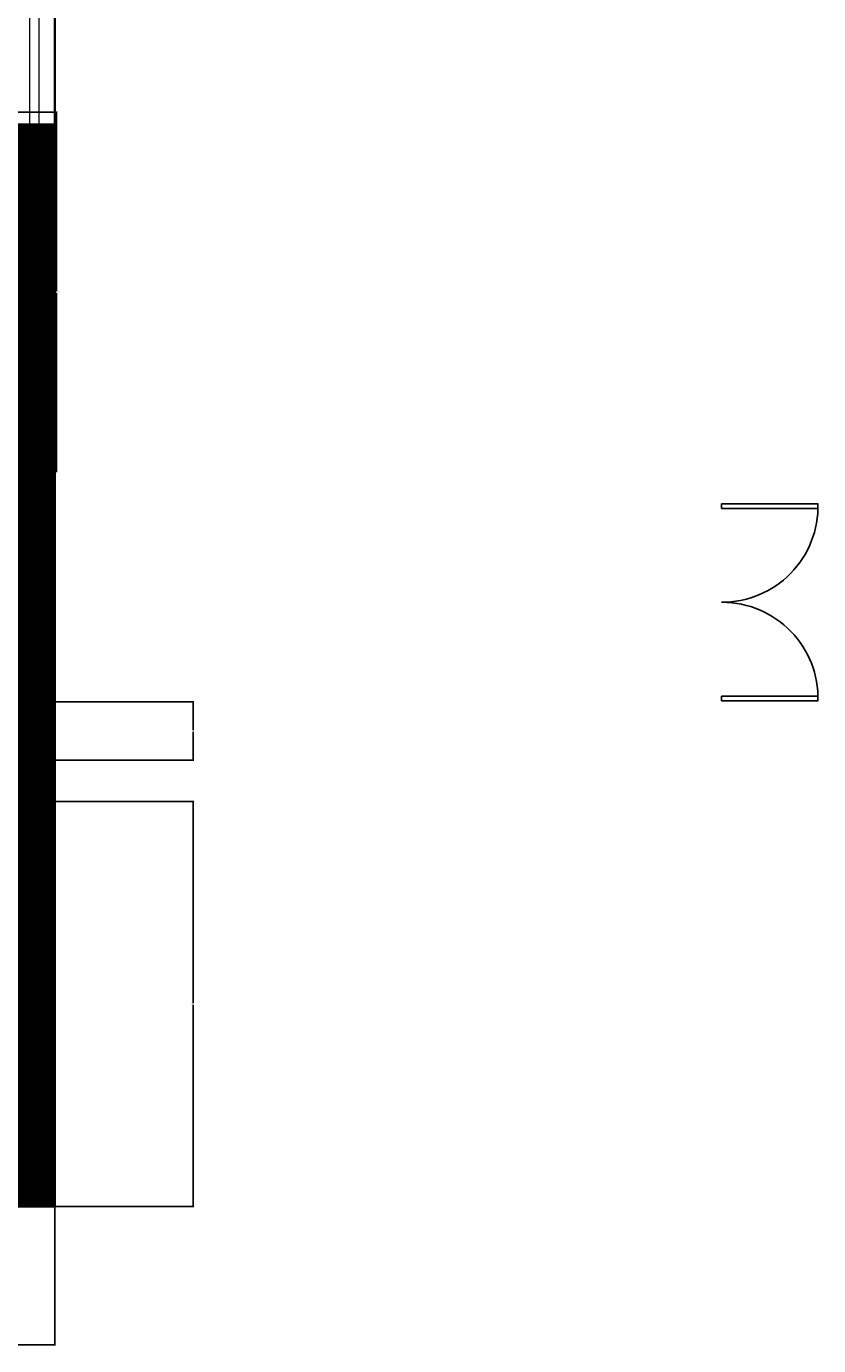
# Model space of a CAD drawing. Units: inches. Extents: x 205 to 1667, y -23 to 828.
# Tile 5 of 10: x 768 to 941, y -23 to 264. Entities that reach past the tile are written whole.
import ezdxf

# ---------------------------------------------------------------- set-up
doc = ezdxf.new("R2010")
doc.units = ezdxf.units.IN
doc.header["$MEASUREMENT"] = 0
for name, color, linetype, lineweight in [('A-ANNO-DIMS', 2, 'Continuous', 18), ('A-DOOR', 4, 'Continuous', 25), ('A-GLAZ', 4, 'Continuous', 18), ('A-WALL', 7, 'Continuous', 35)]:
    doc.layers.add(name, color=color, linetype=linetype, lineweight=lineweight)
doc.layers.add('A-FLOR-PATT', color=9, linetype='Continuous', lineweight=9, true_color=0xc7c8ca)
doc.styles.get("Standard").update_dxf_attribs({"font": 'arial.ttf'})
doc.dimstyles.get("Standard").update_dxf_attribs({"dimtxt": 0.18, "dimasz": 0.18, "dimexe": 0.18, "dimexo": 0.0625, "dimgap": 0.09, "dimtad": 0, "dimtih": 1, "dimtoh": 1, "dimdec": 4, "dimzin": 0, "dimdsep": 46, "dimtxsty": 'Standard', "dimcen": 0.09, "dimadec": 0, "dimazin": 0, "dimtfac": 1, "dimtdec": 4, "dimtofl": 0, "dimtmove": 0, "dimatfit": 3, "dimfxl": 1, "dimtolj": 1, "dimtzin": 0, "dimarcsym": 0})

# ---------------------------------------------------------------- blocks, each defined once
blk = doc.blocks.new('WIN-48IN')
for p, q in [((0, 0), (0, 9)), ((0, 9), (48, 9)), ((48, 9), (48, 0)), ((48, 5.5), (0, 5.5)), ((48, 3.5), (0, 3.5)), ((48, 0), (0, 0))]:
    blk.add_line(p, q)
blk = doc.blocks.new('DOOR-PAIR-21IN-LEAVES')
for p, q in [((0, 42.78), (0, 41.78)), ((0, 42.78), (21, 42.78)), ((0, 41.78), (21, 41.78)), ((0, 1), (0, 0)), ((0, 1), (21, 1)), ((0, 0), (21, 0))]:
    blk.add_line(p, q)
for centre, start, end in [((0.11, 42.28), 269.6873, 1.3714), ((0.11, 0.5), 358.6286, 89.6873)]:
    blk.add_arc(centre, 20.89, start, end)
blk = doc.blocks.new('*D38')
at = {"layer": 'A-ANNO-DIMS', "color": 0, "lineweight": -2, "transparency": 16777216}
for p, q in [((763.1, 245.49), (774.93, 245.49)), ((774.75, 245.31), (774.75, 206.61)), ((774.75, 167.53), (774.75, 206.24)), ((763.1, 167.35), (774.93, 167.35))]:
    blk.add_line(p, q, dxfattribs=at)
at = {"layer": 'A-ANNO-DIMS', "color": 0, "transparency": 16777216}
for points in [[(774.72, 245.31), (774.78, 245.31), (774.75, 245.49)], [(774.72, 167.53), (774.78, 167.53), (774.75, 167.35)]]:
    blk.add_solid(points, dxfattribs=at)
at = {"layer": 'Defpoints', "color": 0, "transparency": 16777216}
for p in [(763.03, 245.49), (763.03, 167.35), (774.75, 167.35)]:
    blk.add_point(p, dxfattribs=at)
at = {"layer": 'A-ANNO-DIMS', "color": 0, "transparency": 16777216, "insert": (774.75, 206.42), "char_height": 0.18, "attachment_point": 5}
blk.add_mtext('\\A1;SOFA 78', dxfattribs=at)
blk = doc.blocks.new('*D42')
at = {"layer": 'A-ANNO-DIMS', "color": 0, "lineweight": -2, "transparency": 16777216}
for p, q in [((462.43, 7.59), (462.43, -22.59)), ((774.43, 7.59), (774.43, -22.59)), ((462.61, -22.41), (618.14, -22.41)), ((774.25, -22.41), (618.72, -22.41))]:
    blk.add_line(p, q, dxfattribs=at)
at = {"layer": 'A-ANNO-DIMS', "color": 0, "transparency": 16777216}
for points in [[(462.61, -22.38), (462.61, -22.44), (462.43, -22.41)], [(774.25, -22.38), (774.25, -22.44), (774.43, -22.41)]]:
    blk.add_solid(points, dxfattribs=at)
at = {"layer": 'Defpoints', "color": 0, "transparency": 16777216}
for p in [(462.43, 7.65), (774.43, 7.65), (774.43, -22.41)]:
    blk.add_point(p, dxfattribs=at)
at = {"layer": 'A-ANNO-DIMS', "color": 0, "transparency": 16777216, "insert": (618.43, -22.41), "char_height": 0.18, "attachment_point": 5}
blk.add_mtext('\\A1;312', dxfattribs=at)
blk = doc.blocks.new('*D45')
at = {"layer": 'A-ANNO-DIMS', "color": 0, "lineweight": -2, "transparency": 16777216}
for p, q in [((765.49, 95.64), (804.67, 95.64)), ((804.49, 95.46), (804.49, 51.83)), ((804.49, 7.83), (804.49, 51.46)), ((774.49, 7.65), (804.67, 7.65))]:
    blk.add_line(p, q, dxfattribs=at)
at = {"layer": 'A-ANNO-DIMS', "color": 0, "transparency": 16777216}
for points in [[(804.46, 95.46), (804.52, 95.46), (804.49, 95.64)], [(804.46, 7.83), (804.52, 7.83), (804.49, 7.65)]]:
    blk.add_solid(points, dxfattribs=at)
at = {"layer": 'Defpoints', "color": 0, "transparency": 16777216}
for p in [(765.43, 95.64), (804.49, 95.64), (774.43, 7.65)]:
    blk.add_point(p, dxfattribs=at)
at = {"layer": 'A-ANNO-DIMS', "color": 0, "transparency": 16777216, "insert": (804.49, 51.64), "char_height": 0.18, "attachment_point": 5}
blk.add_mtext('\\A1;87.99', dxfattribs=at)
blk = doc.blocks.new('*D70')
at = {"layer": 'A-ANNO-DIMS', "color": 0, "lineweight": -2, "transparency": 16777216}
for p, q in [((729.04, 117.32), (804.67, 117.32)), ((804.49, 117.14), (804.49, 111.16)), ((804.49, 104.82), (804.49, 110.8)), ((765.49, 104.64), (804.67, 104.64))]:
    blk.add_line(p, q, dxfattribs=at)
at = {"layer": 'A-ANNO-DIMS', "color": 0, "transparency": 16777216}
for points in [[(804.46, 117.14), (804.52, 117.14), (804.49, 117.32)], [(804.46, 104.82), (804.52, 104.82), (804.49, 104.64)]]:
    blk.add_solid(points, dxfattribs=at)
at = {"layer": 'Defpoints', "color": 0, "transparency": 16777216}
for p in [(728.98, 117.32), (804.49, 117.32), (765.43, 104.64)]:
    blk.add_point(p, dxfattribs=at)
at = {"layer": 'A-ANNO-DIMS', "color": 0, "transparency": 16777216, "insert": (804.49, 110.98), "char_height": 0.18, "attachment_point": 5}
blk.add_mtext('\\A1;12.68', dxfattribs=at)

msp = doc.modelspace()

# ---------------------------------------------------------------- hatches: boundary and pattern name
at = {"layer": 'A-FLOR-PATT'}
h = msp.add_hatch(dxfattribs=at)
h.set_pattern_fill('ANSI31', color=256)
h.paths.add_polyline_path([(774.4305, 607.6511), (720.5338, 607.6511), (720.5338, 598.6511), (727.9933, 598.6511), (746.8614, 598.6511), (765.4305, 598.6511), (765.4305, 454.6511), (759.5298, 454.6511), (759.5298, 448.9635), (765.4305, 448.9635), (765.4305, 428.0602), (774.4305, 428.0602)])
h.paths.add_polyline_path([(765.4305, 598.6511), (746.8614, 598.6511), (746.8614, 579.7829), (727.9933, 579.7829), (727.9933, 518.1387, -0.41421701), (724.6389, 514.7843), (668.2693, 514.7843, -0.41421356), (665.0743, 517.9793), (665.0743, 579.7829), (646.2062, 579.7829), (646.2062, 598.6511), (626.3468, 598.6511), (626.3468, 454.6511), (628.3468, 454.6511), (628.3468, 484.9635, -0.41421356), (664.3468, 449.9635), (664.3468, 454.6511), (729.3305, 454.6511), (758.5298, 454.6511), (759.5298, 454.6511), (765.4305, 454.6511)])
h.paths.add_polyline_path([(621.4404, 598.6511), (471.4305, 598.6511), (471.4305, 568.8442), (490.2987, 568.8442), (490.2987, 549.9761), (551.9429, 549.9761, -0.41421701), (555.2973, 546.6217), (555.2973, 490.2521, -0.41421356), (552.1023, 487.0571), (490.2987, 487.0571), (490.2987, 468.189), (471.4305, 468.189), (471.4305, 454.6511), (583.4404, 454.6511), (583.4404, 449.9635, -0.41421356), (619.4404, 484.9635), (619.4404, 454.6511), (621.4404, 454.6511)])
h.paths.add_polyline_path([(672.5338, 607.6511), (569.5707, 607.6511), (569.5707, 598.6511), (621.4404, 598.6511), (621.4404, 454.6511), (619.4404, 454.6511), (619.4404, 448.9635), (628.3468, 448.9635), (628.3468, 454.6511), (626.3468, 454.6511), (626.3468, 598.6511), (646.2062, 598.6511), (665.0743, 598.6511), (672.5338, 598.6511)])
h.paths.add_polyline_path([(521.5707, 607.6511), (462.4305, 607.6511), (462.4305, 407.4306), (471.4305, 407.4306), (471.4305, 448.9635), (583.4404, 448.9635, -0.0070419), (583.4404, 449.9635), (583.4404, 454.6511), (471.4305, 454.6511), (471.4305, 468.189), (471.4305, 487.0571), (471.4305, 549.9761), (471.4305, 568.8442), (471.4305, 598.6511), (521.5707, 598.6511)])
h.paths.add_polyline_path([(471.4305, 314.3187), (583.4404, 314.3187), (583.4404, 319.9388), (471.4305, 319.9388), (471.4305, 359.4306), (462.4305, 359.4306), (462.4305, 7.6511), (471.4305, 7.6511), (471.4305, 204.9321), (521.9355, 204.9321), (521.9355, 213.9321), (471.4305, 213.9321)])
h.paths.add_polyline_path([(774.4305, 410.0602), (765.4305, 410.0602), (765.4305, 389.1569), (672.3024, 389.1569), (672.3024, 448.9635), (681.1739, 448.9635, -0.18532444), (681.6564, 449.1487), (698.6035, 449.1487), (729.3305, 448.9635), (729.3305, 454.6511), (664.3468, 454.6511), (664.3468, 449.9635, -0.0070419), (664.3468, 448.9635), (666.3024, 448.9635), (666.3024, 378.2485), (672.3024, 378.2485), (672.3024, 383.1306), (765.4305, 383.1306), (765.4305, 360.5347), (774.4305, 360.5347)])
h.paths.add_polyline_path([(774.4305, 342.5347), (765.4305, 342.5347), (765.4305, 319.9388), (672.3024, 319.9388), (672.3024, 348.5574), (671.0896, 348.5574, -0.04071533), (666.3024, 348.2485), (666.3024, 319.9388), (664.3468, 319.9388, -0.0070419), (664.3468, 318.9388), (664.3468, 314.3187), (765.4305, 314.3187), (765.4305, 290.8426), (774.4305, 290.8426)])
h.paths.add_polyline_path([(774.4305, 242.8426), (765.4305, 242.8426), (765.4305, 104.6382), (626.3468, 104.6382), (626.3468, 110.5917), (617.3468, 110.5917), (617.3468, 95.6382), (765.4305, 95.6382), (765.4305, 16.6511), (621.2232, 16.6511), (621.2232, 7.6511), (774.4305, 7.6511)])
h.paths.add_polyline_path([(626.3468, 314.3187), (628.3468, 314.3187), (628.3468, 319.9388), (619.4404, 319.9388), (619.4404, 314.3187), (620.4404, 314.3187), (620.4404, 213.9321), (569.9355, 213.9321), (569.9355, 204.9321), (617.3468, 204.9321), (617.3468, 153.3751), (626.3468, 153.3751)])
h.paths.add_polyline_path([(620.4404, 314.3187), (619.4404, 314.3187), (619.4404, 319.9388), (628.3468, 319.9388), (629.3468, 319.9388), (629.3468, 283.9388, 0.40598745), (664.3468, 318.9388), (664.3468, 319.9388), (666.3024, 319.9388), (666.3024, 348.2485), (666.3024, 377.2485), (666.3024, 378.2485), (666.3024, 448.9635), (664.3468, 448.9635), (664.3468, 449.9635, 0.40598745), (629.3468, 484.9635), (629.3468, 448.9635), (628.3468, 448.9635), (619.4404, 448.9635), (618.4404, 448.9635), (618.4404, 484.9635, 0.40598745), (583.4404, 449.9635), (583.4404, 448.9635), (471.4305, 448.9635), (471.4305, 407.4306), (471.4305, 359.4306), (471.4305, 319.9388), (583.4404, 319.9388), (583.4404, 314.3187), (495.4305, 314.3187), (495.4305, 237.9321), (620.4404, 237.9321)])
h.paths.add_polyline_path([(525.0876, 347.7863), (513.5657, 347.7863), (512.0216, 362.1672), (526.6317, 362.1672)], flags=16)
h.paths.add_polyline_path([(550.9499, 370.1471), (536.569, 368.6029), (536.569, 383.2131), (550.9499, 381.6689)], flags=16)
h.paths.add_polyline_path([(530.7713, 364.5431), (508.0415, 364.5431, -0.41421356), (504.7944, 367.7902), (504.7944, 403.5085, -0.41421356), (508.0415, 406.7556), (530.7713, 406.7556, -0.41421356), (534.0184, 403.5085), (534.0184, 367.7902, -0.41421356)], flags=16)
h.paths.add_polyline_path([(550.9499, 389.6298), (536.569, 388.0856), (536.569, 402.6958), (550.9499, 401.1516)], flags=16)
h.paths.add_polyline_path([(502.2439, 368.6029), (487.863, 370.1471), (487.863, 381.6689), (502.2439, 383.2131)], flags=16)
h.paths.add_polyline_path([(502.2439, 388.0856), (487.863, 389.6298), (487.863, 401.1516), (502.2439, 402.6958)], flags=16)
h.paths.add_polyline_path([(526.6317, 409.1315), (512.0216, 409.1315), (513.5657, 423.5124), (525.0876, 423.5124)], flags=16)
h.paths.add_polyline_path([(765.4305, 290.8426), (765.4305, 314.3187), (664.3468, 314.3187), (664.3468, 318.9388, -0.41421356), (628.3468, 283.9388), (628.3468, 314.3187), (626.3468, 314.3187), (626.3468, 153.3751), (638.3468, 153.3751, -0.4196361), (617.5748, 131.9834, -0.4196361), (638.3468, 110.5917), (626.3468, 110.5917), (626.3468, 104.6382), (765.4305, 104.6382), (765.4305, 242.8426)])
h.paths.add_polyline_path([(691.5064, 243.4363), (693.2483, 243.4363), (725.4984, 243.4363), (725.4984, 241.7329), (725.4984, 177.0512), (723.7564, 177.0512), (691.5064, 177.0512), (691.5064, 178.7545)], flags=16)
h.paths.add_polyline_path([(689.8658, 265.2977), (689.8658, 296.6873, -0.41421356), (690.8346, 297.6561), (724.6111, 297.6561, -0.41421356), (725.5799, 296.6873), (725.5799, 265.2977, -0.41421356), (724.6111, 264.3289), (690.8346, 264.3289, -0.41421356)], flags=16)
h.paths.add_polyline_path([(694.1286, 265.6852), (694.1286, 288.9368, -0.41421356), (695.0974, 289.9056), (720.3483, 289.9056, -0.41421356), (721.3171, 288.9368), (721.3171, 265.6852, -0.04533947), (721.3013, 265.5106, -0.3531705), (720.3282, 264.7164), (695.0974, 264.7164, -0.41421356)], flags=0)
h.paths.add_polyline_path([(694.1286, 291.2619), (694.1286, 294.7497, -0.41421356), (695.0974, 295.7185), (720.3483, 295.7185, -0.41421356), (721.3171, 294.7497), (721.3171, 291.2619, -0.41421356), (720.3483, 290.2931), (695.0974, 290.2931, -0.41421356)], flags=0)
h.paths.add_polyline_path([(734.4369, 244.6615, -0.41421356), (735.2682, 245.4928), (762.2019, 245.4928, -0.41421356), (763.0332, 244.6615), (763.0332, 168.183, -0.41421356), (762.2019, 167.3517), (735.2682, 167.3517, -0.41421356), (734.4369, 168.183)], flags=16)
h.paths.add_polyline_path([(761.7032, 242.1676), (761.7032, 170.6768), (735.6007, 171.0093, -0.41421356), (734.7694, 171.8406), (734.7694, 193.5102, -0.56972741), (735.6007, 194.674, -0.41421356), (734.7694, 195.5053), (734.7694, 217.3423, -0.56972741), (735.6007, 218.5061, -0.41421356), (734.7694, 219.3374), (734.7694, 241.0038, -0.41421356), (735.6007, 241.8351), (735.1643, 242.1676)], flags=16)
h.paths.add_polyline_path([(757.5467, 171.0093), (760.5393, 171.0093, 0.41421356), (761.3706, 171.8406), (761.3706, 193.5102, 0.41421356), (760.5393, 194.3415), (757.5467, 194.3415, 0.41421356), (756.7154, 193.5102), (756.7155, 171.8534, 0.41871477)], flags=0)
h.paths.add_polyline_path([(756.7154, 241.0038, -0.41421356), (757.5467, 241.8351), (760.5393, 241.8351, -0.41421356), (761.3706, 241.0038), (761.3706, 219.3374, -0.41421356), (760.5393, 218.5061), (760.5393, 218.1736, -0.41421356), (761.3706, 217.3423), (761.3706, 195.5053, -0.41421356), (760.5393, 194.674), (757.5467, 194.674, -0.56972741), (756.3829, 195.5053, -0.41421356), (755.5516, 194.674), (755.5516, 194.3415, -0.41421356), (756.3829, 193.5102), (756.7154, 171.8406), (756.3829, 193.5102, 0.41421356), (755.5516, 194.3415), (735.6007, 194.674), (755.5516, 194.674, 0.41421356), (756.3829, 195.5053), (756.3829, 217.3423, 0.41421356), (755.5516, 218.1736), (735.6007, 218.5061), (755.5516, 218.5061, 0.41421356), (756.3829, 219.3374)], flags=0)
h.paths.add_polyline_path([(694.5151, 150.3608), (728.2916, 150.3608, -0.41421356), (729.2604, 149.3919), (729.2604, 118.0023, -0.41421356), (728.2916, 117.0335), (694.5151, 117.0335, -0.41421356), (693.5463, 118.0023), (693.5463, 149.3919, -0.41421356)], flags=16)
h.paths.add_polyline_path([(724.0288, 149.9732, -0.41421356), (724.9977, 149.0044), (724.9977, 125.7529, -0.41421356), (724.0288, 124.784), (698.7779, 124.784, -0.41421356), (697.8091, 125.7529), (697.8091, 149.0044, -0.04533947), (697.825, 149.179, -0.3531705), (698.798, 149.9732)], flags=0)
h.paths.add_polyline_path([(698.7779, 124.3965), (724.0288, 124.3965, -0.41421356), (724.9977, 123.4277), (724.9977, 119.94, -0.41421356), (724.0288, 118.9711), (698.7779, 118.9711, -0.41421356), (697.8091, 119.94), (697.8091, 123.4277, -0.41421356)], flags=0)

# ---------------------------------------------------------------- linework, layer by layer
at = {"layer": 'A-WALL'}
for p, q in [((774.4305, 7.6511), (774.4305, 607.6511)), ((621.2232, 7.6511), (774.4305, 7.6511))]:
    msp.add_line(p, q, dxfattribs=at)

# ---------------------------------------------------------------- block references
at = {"layer": 'A-DOOR'}
msp.add_blockref('DOOR-PAIR-21IN-LEAVES', (919.3922, 117.5739), dxfattribs=at)
at = {"layer": 'A-GLAZ', "rotation": 90.00000000000024}
msp.add_blockref('WIN-48IN', (774.4306, 242.8428), dxfattribs=at)

# ---------------------------------------------------------------- dimensions: what is measured, and where the dimension line sits
at = {"layer": 'A-ANNO-DIMS'}
dim = msp.add_linear_dim(base=(774.7544, 167.3517), p1=(763.0332, 245.4928), p2=(763.0332, 167.3517), angle=270, text='SOFA <>', dimstyle='Standard', override={"dimdec": 0, "dimlfac": 1, "dimrnd": 0, "dimzin": 0, "dimdsep": 46, "dimlunit": 2}, dxfattribs=at)
dim.commit()
dim.dimension.update_dxf_attribs({"geometry": '*D38', "text_midpoint": (774.7544, 206.4222)})
for base, p1, p2, picture, middle in [((804.4881, 117.3173), (765.4305, 104.6382), (728.9767, 117.3173), '*D70', (804.4881, 110.9777)), ((804.4881, 95.6382), (774.4305, 7.6511), (765.4305, 95.6382), '*D45', (804.4881, 51.6446))]:
    dim = msp.add_linear_dim(base=base, p1=p1, p2=p2, angle=90, dimstyle='Standard', override={"dimdec": 2, "dimlfac": 1, "dimrnd": 0, "dimzin": 0, "dimdsep": 46, "dimlunit": 2}, dxfattribs=at)
    dim.commit()
    dim.dimension.update_dxf_attribs({"geometry": picture, "text_midpoint": middle})
dim = msp.add_linear_dim(base=(774.4305, -22.4064), p1=(462.4305, 7.6511), p2=(774.4305, 7.6511), dimstyle='Standard', override={"dimdec": 0, "dimlfac": 1, "dimrnd": 0, "dimzin": 0, "dimdsep": 46, "dimlunit": 2}, dxfattribs=at)
dim.commit()
dim.dimension.update_dxf_attribs({"geometry": '*D42', "text_midpoint": (618.4306, -22.4064)})

doc.saveas('drawing.dxf')
